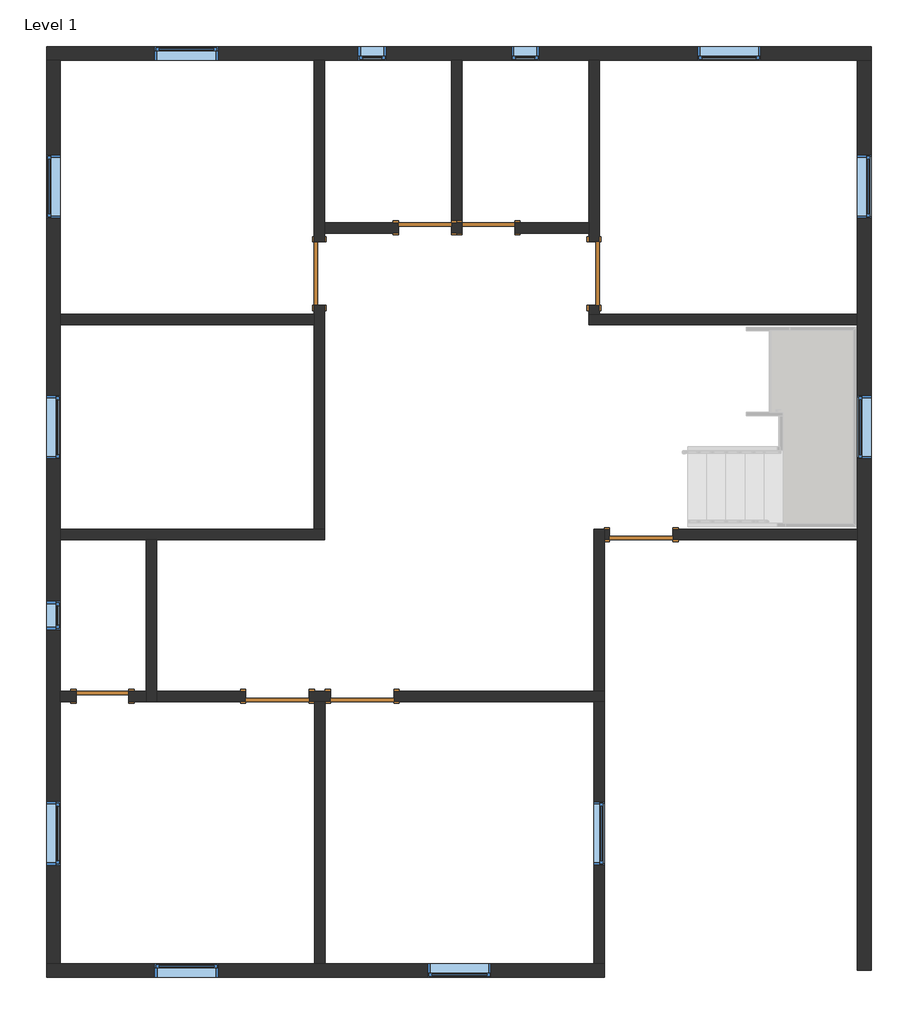
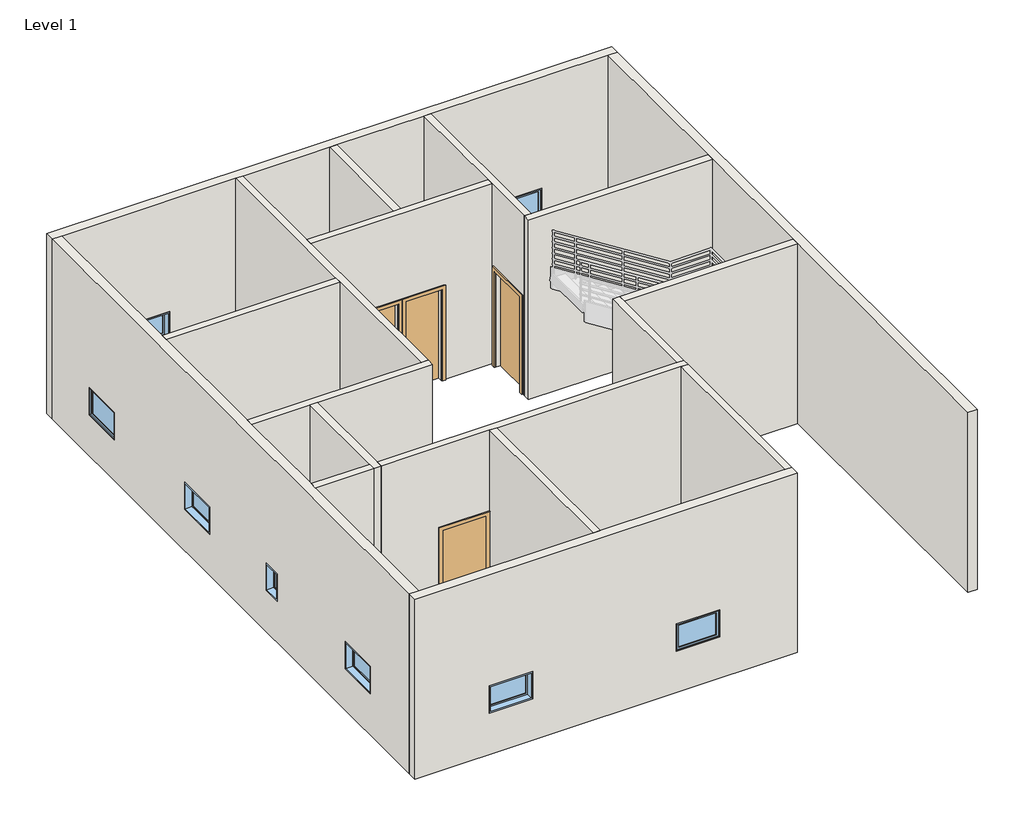
# One storey, part 1 of 3: 18 walls, 13 windows, 8 doors.
"""IFC4 building model written with IfcOpenShell, lengths in millimetres."""

from ifc_helpers import new_model, si_unit, frame, origin, origin_with_axes, place, context, project, spatial, polyline, outline, extrude, faceted_brep, transform, mapped, element, save
from components import m_single_flush_0762_x_2032mm_3f592dcc, m_single_flush_0762_x_2032mm_ffa3ef71, m_single_flush_0915_x_2134mm_f3d7f739, m_single_flush_0915_x_2134mm_138fd904, m_fixed_0406_x_0610mm_8205b201, m_fixed_0915_x_0610mm_70a843a6, m_fixed_0915_x_0610mm_ad787ded

model = new_model("IFC4")

# Units and contexts
model_context = context("Model", 3, world=origin())
ifc_project = project(units=[si_unit("LENGTHUNIT", "METRE", prefix="MILLI")], contexts=[model_context])

# Site, building, storey
site = spatial("IfcSite", under=ifc_project)
building = spatial("IfcBuilding", under=site)
storey = spatial("IfcBuildingStorey", under=building, Name="Level 1", Elevation=0.0)

# Doors
placement = place(None, origin())
m_single_flush_0762_x_2032mm_shape = m_single_flush_0762_x_2032mm_3f592dcc(model_context)
element("IfcDoor", 1, ObjectType="M_Single-Flush : 0762 x 2032mm", at=placement, inside=storey, context=model_context, shape_type="MappedRepresentation", body=[
    mapped(m_single_flush_0762_x_2032mm_shape, transform((-4319.559194, 7327.7632761, 0.0), x_axis=(1.0, 0.0, 0.0), y_axis=(0.0, 1.0, 0.0), z_axis=(0.0, 0.0, 1.0))),
])
m_single_flush_0762_x_2032mm_2_shape = m_single_flush_0762_x_2032mm_ffa3ef71(model_context)
element("IfcDoor", 2, ObjectType="M_Single-Flush : 0762 x 2032mm", at=placement, inside=storey, context=model_context, shape_type="MappedRepresentation", body=[
    mapped(m_single_flush_0762_x_2032mm_2_shape, transform((-3405.159194, 7327.7632761, 0.0), x_axis=(-1.0, 0.0, 0.0), y_axis=(0.0, -1.0, 0.0), z_axis=(0.0, 0.0, 1.0))),
])
element("IfcDoor", 3, ObjectType="M_Single-Flush : 0762 x 2032mm", at=placement, inside=storey, context=model_context, shape_type="MappedRepresentation", body=[
    mapped(m_single_flush_0762_x_2032mm_2_shape, transform((-8968.309194, 576.9132761, 0.0), x_axis=(-1.0, 0.0, 0.0), y_axis=(0.0, -1.0, 0.0), z_axis=(0.0, 0.0, 1.0))),
])
m_single_flush_0915_x_2134mm_shape = m_single_flush_0915_x_2134mm_f3d7f739(model_context)
element("IfcDoor", 4, ObjectType="M_Single-Flush : 0915 x 2134mm", at=placement, inside=storey, context=model_context, shape_type="MappedRepresentation", body=[
    mapped(m_single_flush_0915_x_2134mm_shape, transform((-5841.159194, 6666.3632761, 0.0), x_axis=(0.0, -1.0, 0.0), y_axis=(1.0, 0.0, 0.0), z_axis=(0.0, 0.0, 1.0))),
])
element("IfcDoor", 5, ObjectType="M_Single-Flush : 0915 x 2134mm", at=placement, inside=storey, context=model_context, shape_type="MappedRepresentation", body=[
    mapped(m_single_flush_0915_x_2134mm_shape, transform((-6444.359194, 576.9132761, 0.0), x_axis=(1.0, 0.0, 0.0), y_axis=(0.0, 1.0, 0.0), z_axis=(0.0, 0.0, 1.0))),
])
m_single_flush_0915_x_2134mm_2_shape = m_single_flush_0915_x_2134mm_138fd904(model_context)
element("IfcDoor", 6, ObjectType="M_Single-Flush : 0915 x 2134mm", at=placement, inside=storey, context=model_context, shape_type="MappedRepresentation", body=[
    mapped(m_single_flush_0915_x_2134mm_2_shape, transform((-1881.159194, 6666.3632761, 0.0), x_axis=(0.0, -1.0, 0.0), y_axis=(1.0, 0.0, 0.0), z_axis=(0.0, 0.0, 1.0))),
])
element("IfcDoor", 7, ObjectType="M_Single-Flush : 0915 x 2134mm", at=placement, inside=storey, context=model_context, shape_type="MappedRepresentation", body=[
    mapped(m_single_flush_0915_x_2134mm_2_shape, transform((-5225.159194, 576.9132761, 0.0), x_axis=(-1.0, 0.0, 0.0), y_axis=(0.0, -1.0, 0.0), z_axis=(0.0, 0.0, 1.0))),
])
element("IfcDoor", 8, ObjectType="M_Single-Flush : 0915 x 2134mm", at=placement, inside=storey, context=model_context, shape_type="MappedRepresentation", body=[
    mapped(m_single_flush_0915_x_2134mm_2_shape, transform((-1200.459194, 2907.3632761, 0.0), x_axis=(-1.0, 0.0, 0.0), y_axis=(0.0, -1.0, 0.0), z_axis=(0.0, 0.0, 1.0))),
])

# Walls
element("IfcWall", 9, ObjectType="Generic - 150mm", at=placement, inside=storey, context=model_context, shape_type="SweptSolid", body=[
    extrude(outline(polyline([(-5916.159194, 5929.9632761), (-9573.759194, 5929.9632761), (-9573.759194, 6079.9632761), (-5916.159194, 6079.9632761), (-5916.159194, 5929.9632761)])), origin_with_axes(), (0.0, 0.0, 1.0), 4000.0),
])
element("IfcWall", 10, ObjectType="Generic - 150mm", at=placement, inside=storey, context=model_context, shape_type="Brep", body=[
    faceted_brep([(-5766.159194, 2982.3632761, 0.0), (-5766.159194, 6208.8632761, 0.0), (-5766.159194, 6208.8632761, 2134.0), (-5766.159194, 7123.8632761, 2134.0), (-5766.159194, 7123.8632761, 0.0), (-5766.159194, 7252.7632761, 0.0), (-5766.159194, 7402.7632761, 0.0), (-5766.159194, 9739.1632761, 0.0), (-5766.159194, 9739.1632761, 4000.0), (-5766.159194, 7402.7632761, 4000.0), (-5766.159194, 7252.7632761, 4000.0), (-5766.159194, 2982.3632761, 4000.0), (-5916.159194, 6208.8632761, 2134.0), (-5916.159194, 6208.8632761, 0.0), (-5916.159194, 6079.9632761, 0.0), (-5916.159194, 5929.9632761, 0.0), (-5916.159194, 2982.3632761, 0.0), (-5916.159194, 2982.3632761, 4000.0), (-5916.159194, 5929.9632761, 4000.0), (-5916.159194, 6079.9632761, 4000.0), (-5916.159194, 9739.1632761, 4000.0), (-5916.159194, 9739.1632761, 0.0), (-5916.159194, 7123.8632761, 0.0), (-5916.159194, 7123.8632761, 2134.0)], [[[0, 1, 2, 3, 4, 5, 6, 7, 8, 9, 10, 11]], [[12, 13, 14, 15, 16, 17, 18, 19, 20, 21, 22, 23]], [[22, 21, 7, 6, 5, 4]], [[16, 15, 14, 13, 1, 0]], [[11, 10, 9, 8, 20, 19, 18, 17]], [[8, 7, 21, 20]], [[0, 11, 17, 16]], [[2, 1, 13, 12]], [[3, 2, 12, 23]], [[4, 3, 23, 22]]]),
])
element("IfcWall", 11, ObjectType="Generic - 150mm", at=placement, inside=storey, context=model_context, shape_type="Brep", body=[
    faceted_brep([(-3938.559194, 7252.7632761, 0.0), (-3786.159194, 7252.7632761, 0.0), (-3786.159194, 7252.7632761, 2032.0), (-3024.159194, 7252.7632761, 2032.0), (-3024.159194, 7252.7632761, 0.0), (-1956.159194, 7252.7632761, 0.0), (-1956.159194, 7252.7632761, 4000.0), (-5766.159194, 7252.7632761, 4000.0), (-5766.159194, 7252.7632761, 0.0), (-4700.559194, 7252.7632761, 0.0), (-4700.559194, 7252.7632761, 2032.0), (-3938.559194, 7252.7632761, 2032.0), (-3786.159194, 7402.7632761, 2032.0), (-3786.159194, 7402.7632761, 0.0), (-3787.359194, 7402.7632761, 0.0), (-3937.359194, 7402.7632761, 0.0), (-3938.559194, 7402.7632761, 0.0), (-3938.559194, 7402.7632761, 2032.0), (-4700.559194, 7402.7632761, 2032.0), (-4700.559194, 7402.7632761, 0.0), (-5766.159194, 7402.7632761, 0.0), (-5766.159194, 7402.7632761, 4000.0), (-3937.359194, 7402.7632761, 4000.0), (-3787.359194, 7402.7632761, 4000.0), (-1956.159194, 7402.7632761, 4000.0), (-1956.159194, 7402.7632761, 0.0), (-3024.159194, 7402.7632761, 0.0), (-3024.159194, 7402.7632761, 2032.0)], [[[0, 1, 2, 3, 4, 5, 6, 7, 8, 9, 10, 11]], [[12, 13, 14, 15, 16, 17, 18, 19, 20, 21, 22, 23, 24, 25, 26, 27]], [[9, 8, 20, 19]], [[26, 25, 5, 4]], [[16, 15, 14, 13, 1, 0]], [[7, 6, 24, 23, 22, 21]], [[8, 7, 21, 20]], [[6, 5, 25, 24]], [[17, 16, 0, 11]], [[18, 17, 11, 10]], [[19, 18, 10, 9]], [[2, 1, 13, 12]], [[3, 2, 12, 27]], [[4, 3, 27, 26]]]),
])
element("IfcWall", 12, ObjectType="Generic - 150mm", at=placement, inside=storey, context=model_context, shape_type="SweptSolid", body=[
    extrude(outline(polyline([(-3787.359194, 9739.1632761), (-3787.359194, 7402.7632761), (-3937.359194, 7402.7632761), (-3937.359194, 9739.1632761), (-3787.359194, 9739.1632761)])), origin_with_axes(), (0.0, 0.0, 1.0), 4000.0),
])
element("IfcWall", 13, ObjectType="Generic - 150mm", at=placement, inside=storey, context=model_context, shape_type="Brep", body=[
    faceted_brep([(-1806.159194, 6079.9632761, 0.0), (-1806.159194, 6208.8632761, 0.0), (-1806.159194, 6208.8632761, 2134.0), (-1806.159194, 7123.8632761, 2134.0), (-1806.159194, 7123.8632761, 0.0), (-1806.159194, 9739.1632761, 0.0), (-1806.159194, 9739.1632761, 4000.0), (-1806.159194, 6079.9632761, 4000.0), (-1956.159194, 6208.8632761, 2134.0), (-1956.159194, 6208.8632761, 0.0), (-1956.159194, 6079.9632761, 0.0), (-1956.159194, 6079.9632761, 4000.0), (-1956.159194, 7252.7632761, 4000.0), (-1956.159194, 7402.7632761, 4000.0), (-1956.159194, 9739.1632761, 4000.0), (-1956.159194, 9739.1632761, 0.0), (-1956.159194, 7402.7632761, 0.0), (-1956.159194, 7252.7632761, 0.0), (-1956.159194, 7123.8632761, 0.0), (-1956.159194, 7123.8632761, 2134.0)], [[[0, 1, 2, 3, 4, 5, 6, 7]], [[8, 9, 10, 11, 12, 13, 14, 15, 16, 17, 18, 19]], [[10, 9, 1, 0]], [[18, 17, 16, 15, 5, 4]], [[7, 6, 14, 13, 12, 11]], [[6, 5, 15, 14]], [[0, 7, 11, 10]], [[2, 1, 9, 8]], [[3, 2, 8, 19]], [[4, 3, 19, 18]]]),
])
element("IfcWall", 14, ObjectType="Generic - 150mm", at=placement, inside=storey, context=model_context, shape_type="Brep", body=[
    faceted_brep([(1913.440806, 6079.9632761, 0.0), (-1806.159194, 6079.9632761, 0.0), (-1956.159194, 6079.9632761, 0.0), (-1956.159194, 6079.9632761, 4000.0), (-1806.159194, 6079.9632761, 4000.0), (1913.440806, 6079.9632761, 4000.0), (1913.440806, 5929.9632761, 0.0), (1913.440806, 5929.9632761, 4000.0), (-1956.159194, 5929.9632761, 4000.0), (-1956.159194, 5929.9632761, 0.0)], [[[0, 1, 2, 3, 4, 5]], [[6, 7, 8, 9]], [[2, 1, 0, 6, 9]], [[5, 4, 3, 8, 7]], [[0, 5, 7, 6]], [[3, 2, 9, 8]]]),
])
element("IfcWall", 15, ObjectType="Generic - 150mm", at=placement, inside=storey, context=model_context, shape_type="Brep", body=[
    faceted_brep([(-9573.759194, 2832.3632761, 0.0), (-8337.859194, 2832.3632761, 0.0), (-8187.859194, 2832.3632761, 0.0), (-5766.159194, 2832.3632761, 0.0), (-5766.159194, 2832.3632761, 4000.0), (-8187.859194, 2832.3632761, 4000.0), (-8337.859194, 2832.3632761, 4000.0), (-9573.759194, 2832.3632761, 4000.0), (-9573.759194, 2982.3632761, 0.0), (-9573.759194, 2982.3632761, 4000.0), (-5916.159194, 2982.3632761, 4000.0), (-5766.159194, 2982.3632761, 4000.0), (-5766.159194, 2982.3632761, 0.0), (-5916.159194, 2982.3632761, 0.0)], [[[0, 1, 2, 3, 4, 5, 6, 7]], [[8, 9, 10, 11, 12, 13]], [[3, 2, 1, 0, 8, 13, 12]], [[7, 6, 5, 4, 11, 10, 9]], [[0, 7, 9, 8]], [[4, 3, 12, 11]]]),
])
element("IfcWall", 16, ObjectType="Generic - 150mm", at=placement, inside=storey, context=model_context, shape_type="Brep", body=[
    faceted_brep([(-8337.859194, 2832.3632761, 0.0), (-8337.859194, 651.9132761, 0.0), (-8337.859194, 501.9132761, 0.0), (-8337.859194, 501.9132761, 4000.0), (-8337.859194, 651.9132761, 4000.0), (-8337.859194, 2832.3632761, 4000.0), (-8187.859194, 2832.3632761, 0.0), (-8187.859194, 2832.3632761, 4000.0), (-8187.859194, 651.9132761, 4000.0), (-8187.859194, 501.9132761, 4000.0), (-8187.859194, 501.9132761, 0.0), (-8187.859194, 651.9132761, 0.0)], [[[0, 1, 2, 3, 4, 5]], [[6, 7, 8, 9, 10, 11]], [[2, 1, 0, 6, 11, 10]], [[5, 4, 3, 9, 8, 7]], [[0, 5, 7, 6]], [[3, 2, 10, 9]]]),
])
element("IfcWall", 17, ObjectType="Generic - 150mm", at=placement, inside=storey, context=model_context, shape_type="SweptSolid", body=[
    extrude(outline(polyline([(0.0, -9573.759194), (0.0, -9349.309194), (2032.0, -9349.309194), (2032.0, -8587.309194), (0.0, -8587.309194), (0.0, -8337.859194), (4000.0, -8337.859194), (4000.0, -9573.759194), (0.0, -9573.759194)])), frame((0.0, 501.9132761, 0.0), z_axis=(0.0, 1.0, 0.0), x_axis=(0.0, 0.0, 1.0)), (0.0, 0.0, 1.0), 150.0),
])
element("IfcWall", 18, ObjectType="Generic - 150mm", at=placement, inside=storey, context=model_context, shape_type="Brep", body=[
    faceted_brep([(-5986.859194, 501.9132761, 0.0), (-5909.759194, 501.9132761, 0.0), (-5759.759194, 501.9132761, 0.0), (-5682.659194, 501.9132761, 0.0), (-5682.659194, 501.9132761, 2134.0), (-4767.659194, 501.9132761, 2134.0), (-4767.659194, 501.9132761, 0.0), (-1883.859194, 501.9132761, 0.0), (-1733.859194, 501.9132761, 0.0), (-1733.859194, 501.9132761, 4000.0), (-1883.859194, 501.9132761, 4000.0), (-5759.759194, 501.9132761, 4000.0), (-5909.759194, 501.9132761, 4000.0), (-8187.859194, 501.9132761, 4000.0), (-8187.859194, 501.9132761, 0.0), (-6901.859194, 501.9132761, 0.0), (-6901.859194, 501.9132761, 2134.0), (-5986.859194, 501.9132761, 2134.0), (-5682.659194, 651.9132761, 2134.0), (-5682.659194, 651.9132761, 0.0), (-5986.859194, 651.9132761, 0.0), (-5986.859194, 651.9132761, 2134.0), (-6901.859194, 651.9132761, 2134.0), (-6901.859194, 651.9132761, 0.0), (-8187.859194, 651.9132761, 0.0), (-8187.859194, 651.9132761, 4000.0), (-1885.059194, 651.9132761, 4000.0), (-1735.059194, 651.9132761, 4000.0), (-1733.859194, 651.9132761, 4000.0), (-1733.859194, 651.9132761, 0.0), (-1735.059194, 651.9132761, 0.0), (-1885.059194, 651.9132761, 0.0), (-4767.659194, 651.9132761, 0.0), (-4767.659194, 651.9132761, 2134.0)], [[[0, 1, 2, 3, 4, 5, 6, 7, 8, 9, 10, 11, 12, 13, 14, 15, 16, 17]], [[18, 19, 20, 21, 22, 23, 24, 25, 26, 27, 28, 29, 30, 31, 32, 33]], [[15, 14, 24, 23]], [[20, 19, 3, 2, 1, 0]], [[32, 31, 30, 29, 8, 7, 6]], [[13, 12, 11, 10, 9, 28, 27, 26, 25]], [[14, 13, 25, 24]], [[9, 8, 29, 28]], [[21, 20, 0, 17]], [[22, 21, 17, 16]], [[23, 22, 16, 15]], [[4, 3, 19, 18]], [[5, 4, 18, 33]], [[6, 5, 33, 32]]]),
])
element("IfcWall", 19, ObjectType="Generic - 150mm", at=placement, inside=storey, context=model_context, shape_type="SweptSolid", body=[
    extrude(outline(polyline([(-5909.759194, -3272.0367239), (-5909.759194, 501.9132761), (-5759.759194, 501.9132761), (-5759.759194, -3272.0367239), (-5909.759194, -3272.0367239)])), origin_with_axes(), (0.0, 0.0, 1.0), 4000.0),
])
element("IfcWall", 20, ObjectType="Generic - 150mm", at=placement, inside=storey, context=model_context, shape_type="SweptSolid", body=[
    extrude(outline(polyline([(501.9132761, 0.0), (-3272.0367239, 0.0), (-3272.0367239, 4000.0), (501.9132761, 4000.0), (501.9132761, 0.0)]), holes=[polyline([(-940.0617239, 915.0), (-940.0617239, 1525.0), (-1855.0617239, 1525.0), (-1855.0617239, 915.0), (-940.0617239, 915.0)])]), frame((-1883.859194, 0.0, 0.0), z_axis=(1.0, 0.0, 0.0), x_axis=(0.0, 1.0, 0.0)), (0.0, 0.0, 1.0), 150.0),
])
element("IfcWall", 21, ObjectType="Generic - 150mm", at=placement, inside=storey, context=model_context, shape_type="Brep", body=[
    faceted_brep([(-1735.059194, 651.9132761, 0.0), (-1735.059194, 2832.3632761, 0.0), (-1735.059194, 2982.3632761, 0.0), (-1735.059194, 2982.3632761, 4000.0), (-1735.059194, 2832.3632761, 4000.0), (-1735.059194, 651.9132761, 4000.0), (-1885.059194, 651.9132761, 0.0), (-1885.059194, 651.9132761, 4000.0), (-1885.059194, 2982.3632761, 4000.0), (-1885.059194, 2982.3632761, 0.0)], [[[0, 1, 2, 3, 4, 5]], [[6, 7, 8, 9]], [[2, 1, 0, 6, 9]], [[5, 4, 3, 8, 7]], [[0, 5, 7, 6]], [[3, 2, 9, 8]]]),
])
element("IfcWall", 22, ObjectType="Generic - 150mm", at=placement, inside=storey, context=model_context, shape_type="SweptSolid", body=[
    extrude(outline(polyline([(0.0, -1735.059194), (0.0, -1657.959194), (2134.0, -1657.959194), (2134.0, -742.959194), (0.0, -742.959194), (0.0, 1913.440806), (4000.0, 1913.440806), (4000.0, -1735.059194), (0.0, -1735.059194)])), frame((0.0, 2832.3632761, 0.0), z_axis=(0.0, 1.0, 0.0), x_axis=(0.0, 0.0, 1.0)), (0.0, 0.0, 1.0), 150.0),
])
element("IfcWall", 23, ObjectType="Generic - 200mm", at=placement, inside=storey, context=model_context, shape_type="Brep", body=[
    faceted_brep([(-9773.759194, 9739.1632761, 0.0), (-9573.759194, 9739.1632761, 0.0), (-5916.159194, 9739.1632761, 0.0), (-5766.159194, 9739.1632761, 0.0), (-3937.359194, 9739.1632761, 0.0), (-3787.359194, 9739.1632761, 0.0), (-1956.159194, 9739.1632761, 0.0), (-1806.159194, 9739.1632761, 0.0), (1913.440806, 9739.1632761, 0.0), (2113.440806, 9739.1632761, 0.0), (2113.440806, 9739.1632761, 4000.0), (1913.440806, 9739.1632761, 4000.0), (-1806.159194, 9739.1632761, 4000.0), (-1956.159194, 9739.1632761, 4000.0), (-3787.359194, 9739.1632761, 4000.0), (-3937.359194, 9739.1632761, 4000.0), (-5766.159194, 9739.1632761, 4000.0), (-5916.159194, 9739.1632761, 4000.0), (-9573.759194, 9739.1632761, 4000.0), (-9773.759194, 9739.1632761, 4000.0), (-4876.159194, 9739.1632761, 915.0), (-5282.159194, 9739.1632761, 915.0), (-5282.159194, 9739.1632761, 1525.0), (-4876.159194, 9739.1632761, 1525.0), (-2668.759194, 9739.1632761, 915.0), (-3074.759194, 9739.1632761, 915.0), (-3074.759194, 9739.1632761, 1525.0), (-2668.759194, 9739.1632761, 1525.0), (-8214.959194, 9739.1632761, 915.0), (-8214.959194, 9739.1632761, 1525.0), (-7299.959194, 9739.1632761, 1525.0), (-7299.959194, 9739.1632761, 915.0), (523.640806, 9739.1632761, 915.0), (-391.359194, 9739.1632761, 915.0), (-391.359194, 9739.1632761, 1525.0), (523.640806, 9739.1632761, 1525.0), (-9773.759194, 9939.1632761, 0.0), (-9773.759194, 9939.1632761, 4000.0), (2113.440806, 9939.1632761, 4000.0), (2113.440806, 9939.1632761, 0.0), (-4876.159194, 9939.1632761, 915.0), (-4876.159194, 9939.1632761, 1525.0), (-5282.159194, 9939.1632761, 1525.0), (-5282.159194, 9939.1632761, 915.0), (-2668.759194, 9939.1632761, 915.0), (-2668.759194, 9939.1632761, 1525.0), (-3074.759194, 9939.1632761, 1525.0), (-3074.759194, 9939.1632761, 915.0), (-8214.959194, 9939.1632761, 915.0), (-7299.959194, 9939.1632761, 915.0), (-7299.959194, 9939.1632761, 1525.0), (-8214.959194, 9939.1632761, 1525.0), (523.640806, 9939.1632761, 915.0), (523.640806, 9939.1632761, 1525.0), (-391.359194, 9939.1632761, 1525.0), (-391.359194, 9939.1632761, 915.0)], [[[0, 1, 2, 3, 4, 5, 6, 7, 8, 9, 10, 11, 12, 13, 14, 15, 16, 17, 18, 19], [20, 21, 22, 23], [24, 25, 26, 27], [28, 29, 30, 31], [32, 33, 34, 35]], [[36, 37, 38, 39], [40, 41, 42, 43], [44, 45, 46, 47], [48, 49, 50, 51], [52, 53, 54, 55]], [[9, 8, 7, 6, 5, 4, 3, 2, 1, 0, 36, 39]], [[19, 18, 17, 16, 15, 14, 13, 12, 11, 10, 38, 37]], [[10, 9, 39, 38]], [[0, 19, 37, 36]], [[41, 40, 20, 23]], [[42, 41, 23, 22]], [[43, 42, 22, 21]], [[40, 43, 21, 20]], [[45, 44, 24, 27]], [[46, 45, 27, 26]], [[47, 46, 26, 25]], [[44, 47, 25, 24]], [[29, 28, 48, 51]], [[30, 29, 51, 50]], [[31, 30, 50, 49]], [[28, 31, 49, 48]], [[53, 52, 32, 35]], [[54, 53, 35, 34]], [[55, 54, 34, 33]], [[52, 55, 33, 32]]]),
])
element("IfcWall", 24, ObjectType="Generic - 200mm", at=placement, inside=storey, context=model_context, shape_type="Brep", body=[
    faceted_brep([(1913.440806, 9739.1632761, 0.0), (1913.440806, 6079.9632761, 0.0), (1913.440806, 5929.9632761, 0.0), (1913.440806, 2982.3632761, 0.0), (1913.440806, 2832.3632761, 0.0), (1913.440806, -3372.0367239, 0.0), (1913.440806, -3372.0367239, 4000.0), (1913.440806, 2832.3632761, 4000.0), (1913.440806, 2982.3632761, 4000.0), (1913.440806, 5929.9632761, 4000.0), (1913.440806, 6079.9632761, 4000.0), (1913.440806, 9739.1632761, 4000.0), (1913.440806, 8379.5632761, 915.0), (1913.440806, 8379.5632761, 1525.0), (1913.440806, 7464.5632761, 1525.0), (1913.440806, 7464.5632761, 915.0), (1913.440806, 3998.6632761, 915.0), (1913.440806, 4913.6632761, 915.0), (1913.440806, 4913.6632761, 1525.0), (1913.440806, 3998.6632761, 1525.0), (2113.440806, 9739.1632761, 0.0), (2113.440806, 9739.1632761, 4000.0), (2113.440806, -3372.0367239, 4000.0), (2113.440806, -3372.0367239, 0.0), (2113.440806, 8379.5632761, 915.0), (2113.440806, 7464.5632761, 915.0), (2113.440806, 7464.5632761, 1525.0), (2113.440806, 8379.5632761, 1525.0), (2113.440806, 3998.6632761, 915.0), (2113.440806, 3998.6632761, 1525.0), (2113.440806, 4913.6632761, 1525.0), (2113.440806, 4913.6632761, 915.0)], [[[0, 1, 2, 3, 4, 5, 6, 7, 8, 9, 10, 11], [12, 13, 14, 15], [16, 17, 18, 19]], [[20, 21, 22, 23], [24, 25, 26, 27], [28, 29, 30, 31]], [[5, 4, 3, 2, 1, 0, 20, 23]], [[6, 5, 23, 22]], [[11, 10, 9, 8, 7, 6, 22, 21]], [[0, 11, 21, 20]], [[13, 12, 24, 27]], [[14, 13, 27, 26]], [[15, 14, 26, 25]], [[12, 15, 25, 24]], [[29, 28, 16, 19]], [[30, 29, 19, 18]], [[31, 30, 18, 17]], [[28, 31, 17, 16]]]),
])
element("IfcWall", 25, ObjectType="Generic - 200mm", at=placement, inside=storey, context=model_context, shape_type="Brep", body=[
    faceted_brep([(-1733.859194, -3272.0367239, 0.0), (-1883.859194, -3272.0367239, 0.0), (-5759.759194, -3272.0367239, 0.0), (-5909.759194, -3272.0367239, 0.0), (-9573.759194, -3272.0367239, 0.0), (-9773.759194, -3272.0367239, 0.0), (-9773.759194, -3272.0367239, 4000.0), (-9573.759194, -3272.0367239, 4000.0), (-5909.759194, -3272.0367239, 4000.0), (-5759.759194, -3272.0367239, 4000.0), (-1883.859194, -3272.0367239, 4000.0), (-1733.859194, -3272.0367239, 4000.0), (-3364.309194, -3272.0367239, 915.0), (-3364.309194, -3272.0367239, 1525.0), (-4279.309194, -3272.0367239, 1525.0), (-4279.309194, -3272.0367239, 915.0), (-8211.759194, -3272.0367239, 915.0), (-7296.759194, -3272.0367239, 915.0), (-7296.759194, -3272.0367239, 1525.0), (-8211.759194, -3272.0367239, 1525.0), (-1733.859194, -3472.0367239, 0.0), (-1733.859194, -3472.0367239, 4000.0), (-9773.759194, -3472.0367239, 4000.0), (-9773.759194, -3472.0367239, 0.0), (-3364.309194, -3472.0367239, 915.0), (-4279.309194, -3472.0367239, 915.0), (-4279.309194, -3472.0367239, 1525.0), (-3364.309194, -3472.0367239, 1525.0), (-8211.759194, -3472.0367239, 915.0), (-8211.759194, -3472.0367239, 1525.0), (-7296.759194, -3472.0367239, 1525.0), (-7296.759194, -3472.0367239, 915.0)], [[[0, 1, 2, 3, 4, 5, 6, 7, 8, 9, 10, 11], [12, 13, 14, 15], [16, 17, 18, 19]], [[20, 21, 22, 23], [24, 25, 26, 27], [28, 29, 30, 31]], [[5, 4, 3, 2, 1, 0, 20, 23]], [[11, 10, 9, 8, 7, 6, 22, 21]], [[6, 5, 23, 22]], [[13, 12, 24, 27]], [[14, 13, 27, 26]], [[15, 14, 26, 25]], [[12, 15, 25, 24]], [[29, 28, 16, 19]], [[30, 29, 19, 18]], [[31, 30, 18, 17]], [[28, 31, 17, 16]], [[0, 11, 21, 20]]]),
])
element("IfcWall", 26, ObjectType="Generic - 200mm", at=placement, inside=storey, context=model_context, shape_type="Brep", body=[
    faceted_brep([(-9573.759194, -3272.0367239, 0.0), (-9573.759194, 501.9132761, 0.0), (-9573.759194, 651.9132761, 0.0), (-9573.759194, 2832.3632761, 0.0), (-9573.759194, 2982.3632761, 0.0), (-9573.759194, 5929.9632761, 0.0), (-9573.759194, 6079.9632761, 0.0), (-9573.759194, 9739.1632761, 0.0), (-9573.759194, 9739.1632761, 4000.0), (-9573.759194, 6079.9632761, 4000.0), (-9573.759194, 5929.9632761, 4000.0), (-9573.759194, 2982.3632761, 4000.0), (-9573.759194, 2832.3632761, 4000.0), (-9573.759194, 651.9132761, 4000.0), (-9573.759194, 501.9132761, 4000.0), (-9573.759194, -3272.0367239, 4000.0), (-9573.759194, 1945.1382761, 915.0), (-9573.759194, 1539.1382761, 915.0), (-9573.759194, 1539.1382761, 1525.0), (-9573.759194, 1945.1382761, 1525.0), (-9573.759194, 7464.5632761, 915.0), (-9573.759194, 7464.5632761, 1525.0), (-9573.759194, 8379.5632761, 1525.0), (-9573.759194, 8379.5632761, 915.0), (-9573.759194, -940.0617239, 915.0), (-9573.759194, -1855.0617239, 915.0), (-9573.759194, -1855.0617239, 1525.0), (-9573.759194, -940.0617239, 1525.0), (-9573.759194, 4913.6632761, 915.0), (-9573.759194, 3998.6632761, 915.0), (-9573.759194, 3998.6632761, 1525.0), (-9573.759194, 4913.6632761, 1525.0), (-9773.759194, -3272.0367239, 0.0), (-9773.759194, -3272.0367239, 4000.0), (-9773.759194, 9739.1632761, 4000.0), (-9773.759194, 9739.1632761, 0.0), (-9773.759194, 1945.1382761, 915.0), (-9773.759194, 1945.1382761, 1525.0), (-9773.759194, 1539.1382761, 1525.0), (-9773.759194, 1539.1382761, 915.0), (-9773.759194, 7464.5632761, 915.0), (-9773.759194, 8379.5632761, 915.0), (-9773.759194, 8379.5632761, 1525.0), (-9773.759194, 7464.5632761, 1525.0), (-9773.759194, -940.0617239, 915.0), (-9773.759194, -940.0617239, 1525.0), (-9773.759194, -1855.0617239, 1525.0), (-9773.759194, -1855.0617239, 915.0), (-9773.759194, 4913.6632761, 915.0), (-9773.759194, 4913.6632761, 1525.0), (-9773.759194, 3998.6632761, 1525.0), (-9773.759194, 3998.6632761, 915.0)], [[[0, 1, 2, 3, 4, 5, 6, 7, 8, 9, 10, 11, 12, 13, 14, 15], [16, 17, 18, 19], [20, 21, 22, 23], [24, 25, 26, 27], [28, 29, 30, 31]], [[32, 33, 34, 35], [36, 37, 38, 39], [40, 41, 42, 43], [44, 45, 46, 47], [48, 49, 50, 51]], [[7, 6, 5, 4, 3, 2, 1, 0, 32, 35]], [[15, 14, 13, 12, 11, 10, 9, 8, 34, 33]], [[8, 7, 35, 34]], [[0, 15, 33, 32]], [[37, 36, 16, 19]], [[38, 37, 19, 18]], [[39, 38, 18, 17]], [[36, 39, 17, 16]], [[21, 20, 40, 43]], [[22, 21, 43, 42]], [[23, 22, 42, 41]], [[20, 23, 41, 40]], [[45, 44, 24, 27]], [[46, 45, 27, 26]], [[47, 46, 26, 25]], [[44, 47, 25, 24]], [[49, 48, 28, 31]], [[50, 49, 31, 30]], [[51, 50, 30, 29]], [[48, 51, 29, 28]]]),
])

# Windows
m_fixed_0406_x_0610mm_shape = m_fixed_0406_x_0610mm_8205b201(model_context)
element("IfcWindow", 27, ObjectType="M_Fixed : 0406 x 0610mm", at=placement, inside=storey, context=model_context, shape_type="MappedRepresentation", body=[
    mapped(m_fixed_0406_x_0610mm_shape, transform((-5079.159194, 9852.1632761, 0.0), x_axis=(-1.0, 0.0, 0.0), y_axis=(0.0, -1.0, 0.0), z_axis=(0.0, 0.0, 1.0))),
])
element("IfcWindow", 28, ObjectType="M_Fixed : 0406 x 0610mm", at=placement, inside=storey, context=model_context, shape_type="MappedRepresentation", body=[
    mapped(m_fixed_0406_x_0610mm_shape, transform((-2871.759194, 9852.1632761, 0.0), x_axis=(-1.0, 0.0, 0.0), y_axis=(0.0, -1.0, 0.0), z_axis=(0.0, 0.0, 1.0))),
])
element("IfcWindow", 29, ObjectType="M_Fixed : 0406 x 0610mm", at=placement, inside=storey, context=model_context, shape_type="MappedRepresentation", body=[
    mapped(m_fixed_0406_x_0610mm_shape, transform((-9686.759194, 1742.1382761, 0.0), x_axis=(0.0, -1.0, 0.0), y_axis=(1.0, 0.0, 0.0), z_axis=(0.0, 0.0, 1.0))),
])
m_fixed_0915_x_0610mm_shape = m_fixed_0915_x_0610mm_70a843a6(model_context)
element("IfcWindow", 30, ObjectType="M_Fixed : 0915 x 0610mm", at=placement, inside=storey, context=model_context, shape_type="MappedRepresentation", body=[
    mapped(m_fixed_0915_x_0610mm_shape, transform((-9660.759194, 7922.0632761, 0.0), x_axis=(0.0, 1.0, 0.0), y_axis=(-1.0, 0.0, 0.0), z_axis=(0.0, 0.0, 1.0))),
])
element("IfcWindow", 31, ObjectType="M_Fixed : 0915 x 0610mm", at=placement, inside=storey, context=model_context, shape_type="MappedRepresentation", body=[
    mapped(m_fixed_0915_x_0610mm_shape, transform((-7757.459194, 9826.1632761, 0.0), x_axis=(1.0, 0.0, 0.0), y_axis=(0.0, 1.0, 0.0), z_axis=(0.0, 0.0, 1.0))),
])
element("IfcWindow", 32, ObjectType="M_Fixed : 0915 x 0610mm", at=placement, inside=storey, context=model_context, shape_type="MappedRepresentation", body=[
    mapped(m_fixed_0915_x_0610mm_shape, transform((66.140806, 9852.1632761, 0.0), x_axis=(-1.0, 0.0, 0.0), y_axis=(0.0, -1.0, 0.0), z_axis=(0.0, 0.0, 1.0))),
])
element("IfcWindow", 33, ObjectType="M_Fixed : 0915 x 0610mm", at=placement, inside=storey, context=model_context, shape_type="MappedRepresentation", body=[
    mapped(m_fixed_0915_x_0610mm_shape, transform((2000.440806, 7922.0632761, 0.0), x_axis=(0.0, -1.0, 0.0), y_axis=(1.0, 0.0, 0.0), z_axis=(0.0, 0.0, 1.0))),
])
element("IfcWindow", 34, ObjectType="M_Fixed : 0915 x 0610mm", at=placement, inside=storey, context=model_context, shape_type="MappedRepresentation", body=[
    mapped(m_fixed_0915_x_0610mm_shape, transform((2026.440806, 4456.1632761, 0.0), x_axis=(0.0, 1.0, 0.0), y_axis=(-1.0, 0.0, 0.0), z_axis=(0.0, 0.0, 1.0))),
])
element("IfcWindow", 35, ObjectType="M_Fixed : 0915 x 0610mm", at=placement, inside=storey, context=model_context, shape_type="MappedRepresentation", body=[
    mapped(m_fixed_0915_x_0610mm_shape, transform((-3821.809194, -3359.0367239, 0.0), x_axis=(-1.0, 0.0, 0.0), y_axis=(0.0, -1.0, 0.0), z_axis=(0.0, 0.0, 1.0))),
])
element("IfcWindow", 36, ObjectType="M_Fixed : 0915 x 0610mm", at=placement, inside=storey, context=model_context, shape_type="MappedRepresentation", body=[
    mapped(m_fixed_0915_x_0610mm_shape, transform((-7754.259194, -3385.0367239, 0.0), x_axis=(1.0, 0.0, 0.0), y_axis=(0.0, 1.0, 0.0), z_axis=(0.0, 0.0, 1.0))),
])
element("IfcWindow", 37, ObjectType="M_Fixed : 0915 x 0610mm", at=placement, inside=storey, context=model_context, shape_type="MappedRepresentation", body=[
    mapped(m_fixed_0915_x_0610mm_shape, transform((-9686.759194, -1397.5617239, 0.0), x_axis=(0.0, -1.0, 0.0), y_axis=(1.0, 0.0, 0.0), z_axis=(0.0, 0.0, 1.0))),
])
element("IfcWindow", 38, ObjectType="M_Fixed : 0915 x 0610mm", at=placement, inside=storey, context=model_context, shape_type="MappedRepresentation", body=[
    mapped(m_fixed_0915_x_0610mm_shape, transform((-9686.759194, 4456.1632761, 0.0), x_axis=(0.0, -1.0, 0.0), y_axis=(1.0, 0.0, 0.0), z_axis=(0.0, 0.0, 1.0))),
])
m_fixed_0915_x_0610mm_2_shape = m_fixed_0915_x_0610mm_ad787ded(model_context)
element("IfcWindow", 39, ObjectType="M_Fixed : 0915 x 0610mm", at=placement, inside=storey, context=model_context, shape_type="MappedRepresentation", body=[
    mapped(m_fixed_0915_x_0610mm_2_shape, transform((-1821.859194, -1397.5617239, 0.0), x_axis=(0.0, -1.0, 0.0), y_axis=(1.0, 0.0, 0.0), z_axis=(0.0, 0.0, 1.0))),
])

save(model, "model.ifc")

# Revit data of these elements
# Type "M_Single-Flush : 0762 x 2032mm"
#   Type Mark = "19"
#   Thickness = 51 mm
#   Height = 2032 mm
#   Trim Projection Ext = 25 mm
#   Trim Projection Int = 25 mm
#   Trim Width = 76 mm
#   Width = 762 mm
#   Door Material = Door - Panel
#   Frame Material = Door - Frame
#   Function = (empty or 0)
#   Wall Closure = (empty or 0)
# Type "M_Single-Flush : 0915 x 2134mm"
#   Type Mark = "15"
#   Thickness = 51 mm
#   Height = 2134 mm
#   Trim Projection Ext = 25 mm
#   Trim Projection Int = 25 mm
#   Trim Width = 76 mm
#   Width = 915 mm
#   Door Material = Door - Panel
#   Frame Material = Door - Frame
#   Function = (empty or 0)
#   Wall Closure = (empty or 0)
# Type "Generic - 150mm"
#   Layers, outside or top first: 150 mm no material (function 1)
# Type "Generic - 200mm"
#   Layers, outside or top first: 200 mm no material (function 1)
# Type "M_Fixed : 0406 x 0610mm"
#   Type Mark = "10"
#   Height = 610 mm
#   Default Sill Height = 915 mm
#   Width = 406 mm
#   Window Inset = 19 mm
#   Frame Exterior Material = Sash
#   Frame Interior Material = Sash
#   Glass Pane Material = Glass
#   Sash = Sash
#   Wall Closure = (empty or 0)
# Type "M_Fixed : 0915 x 0610mm"
#   Type Mark = "14"
#   Height = 610 mm
#   Default Sill Height = 915 mm
#   Width = 915 mm
#   Window Inset = 19 mm
#   Frame Exterior Material = Sash
#   Frame Interior Material = Sash
#   Glass Pane Material = Glass
#   Sash = Sash
#   Wall Closure = (empty or 0)
# Elements 1, 2, 3 (IfcDoor, "M_Single-Flush : 0762 x 2032mm")
#   Phase Created = New Construction
#   Materials on its faces: "Door - Frame", "Door - Panel"
# Elements 4, 5, 6, 7, 8 (IfcDoor, "M_Single-Flush : 0915 x 2134mm")
#   Phase Created = New Construction
#   Materials on its faces: "Door - Frame", "Door - Panel"
# Elements 9, 10, 11, 12, 13, 14, 15, 16, 17, 18, 19, 20, 21, 22 (IfcWall, "Generic - 150mm")
#   Top Offset = 0 mm
#   Base Offset = 0 mm
#   wall height = 4000 mm
#   Phase Created = New Construction
#   Base Constraint = Level 1
#   Top Constraint = Level 2
#   Materials on its faces: "Default Wall"
# Elements 23, 24, 25, 26 (IfcWall, "Generic - 200mm")
#   Top Offset = 0 mm
#   Base Offset = 0 mm
#   wall height = 4000 mm
#   Phase Created = New Construction
#   Base Constraint = Level 1
#   Top Constraint = Level 2
#   Materials on its faces: "Default Wall"
# Element 27 (IfcWindow, "M_Fixed : 0406 x 0610mm")
#   Mark = "6"
#   Phase Created = New Construction
#   Materials on its faces: "Sash", "Glass"
# Element 28 (IfcWindow, "M_Fixed : 0406 x 0610mm")
#   Mark = "7"
#   Phase Created = New Construction
#   Materials on its faces: "Sash", "Glass"
# Element 29 (IfcWindow, "M_Fixed : 0406 x 0610mm")
#   Mark = "8"
#   Phase Created = New Construction
#   Materials on its faces: "Sash", "Glass"
# Element 30 (IfcWindow, "M_Fixed : 0915 x 0610mm")
#   Mark = "9"
#   Phase Created = New Construction
#   Materials on its faces: "Sash", "Glass"
# Element 31 (IfcWindow, "M_Fixed : 0915 x 0610mm")
#   Mark = "10"
#   Phase Created = New Construction
#   Materials on its faces: "Sash", "Glass"
# Element 32 (IfcWindow, "M_Fixed : 0915 x 0610mm")
#   Mark = "11"
#   Phase Created = New Construction
#   Materials on its faces: "Sash", "Glass"
# Element 33 (IfcWindow, "M_Fixed : 0915 x 0610mm")
#   Mark = "12"
#   Phase Created = New Construction
#   Materials on its faces: "Sash", "Glass"
# Element 34 (IfcWindow, "M_Fixed : 0915 x 0610mm")
#   Mark = "13"
#   Phase Created = New Construction
#   Materials on its faces: "Sash", "Glass"
# Element 35 (IfcWindow, "M_Fixed : 0915 x 0610mm")
#   Mark = "15"
#   Phase Created = New Construction
#   Materials on its faces: "Sash", "Glass"
# Element 36 (IfcWindow, "M_Fixed : 0915 x 0610mm")
#   Mark = "16"
#   Phase Created = New Construction
#   Materials on its faces: "Sash", "Glass"
# Element 37 (IfcWindow, "M_Fixed : 0915 x 0610mm")
#   Mark = "17"
#   Phase Created = New Construction
#   Materials on its faces: "Sash", "Glass"
# Element 38 (IfcWindow, "M_Fixed : 0915 x 0610mm")
#   Mark = "18"
#   Phase Created = New Construction
#   Materials on its faces: "Sash", "Glass"
# Element 39 (IfcWindow, "M_Fixed : 0915 x 0610mm")
#   Mark = "14"
#   Phase Created = New Construction
#   Materials on its faces: "Sash", "Glass"
# Materials
#   "Door - Panel": class "Wood", colour RGB 114 82 51, transparency 0
#   "Door - Frame": colour RGB 153 76 43, transparency 0
#   "Sash": class "Wood", colour RGB 136 99 55, transparency 0
#   "Glass": class "Glass", colour RGB 218 227 224, transparency 0.85, Description = "Soda Lime Glass", Cost = 0
#   "Default Wall": colour RGB 80 80 80, transparency 0
